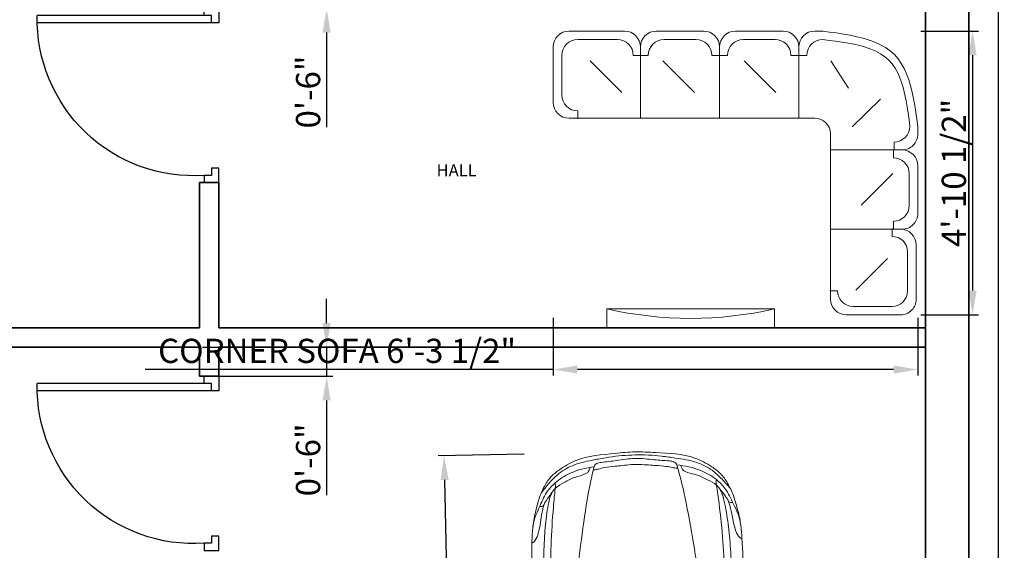
# Model space of a CAD drawing. Units: inches. Extents: x -24887 to 3061, y 1794 to 4919553.
# Tile 11 of 14: x 2858 to 3061, y 2080 to 2190. Entities that reach past the tile are written whole.
import ezdxf

# ---------------------------------------------------------------- set-up
doc = ezdxf.new("R2010")
doc.units = ezdxf.units.IN
for name, color, linetype, lineweight in [('A-ANNO-DIMS', 2, 'Continuous', 18), ('A-AREA-IDEN', 7, 'Continuous', 18), ('A-FLOR-PRKG', 8, 'Continuous', 13), ('A-FURN', 8, 'Continuous', 18), ('door', 4, 'Continuous', 25), ('TV', 210, 'Continuous', 18), ('wall', 7, 'Continuous', 35)]:
    doc.layers.add(name, color=color, linetype=linetype, lineweight=lineweight)
doc.styles.get("Standard").update_dxf_attribs({"font": 'arial.ttf'})
doc.dimstyles.new('ISO-25', dxfattribs={"dimtxt": 5, "dimasz": 5, "dimexe": 1.25, "dimexo": 0.625, "dimtad": 1, "dimdec": 1, "dimlunit": 3, "dimtxsty": 'Standard', "dimcen": 2.5, "dimadec": 0, "dimazin": 0, "dimtfac": 1, "dimtdec": 1, "dimtmove": 0, "dimatfit": 3, "dimfxl": 1, "dimarcsym": 0})

# ---------------------------------------------------------------- blocks, each defined once
blk = doc.blocks.new('A$C242571DA')
for points, knots in [([(0, 873.4), (0, 927.8), (15.6, 1088.6), (25.5, 1309.8), (120.7, 1476.4), (189.2, 1569), (273.5, 1623.1), (369.9, 1666.3), (483, 1694.7), (561.3, 1714.9), (604.6, 1715.7)], [0, 0, 0, 0, 0.16039, 0.479033, 0.632967, 0.722015, 0.817474, 0.927562, 1.03733, 1.167094, 1.167094, 1.167094, 1.167094]), ([(604.6, 1715.7), (545.5, 1714.5), (448.5, 1664.6), (320.8, 1610.6), (225.4, 1521.2), (147.3, 1390.5), (121.7, 1275.2), (113.6, 1208.7)], [0, 0, 0, 0, 0.1772572, 0.3124951, 0.4151678, 0.5597243, 0.7575412, 0.7575412, 0.7575412, 0.7575412]), ([(722.7, 1726.6), (720.8, 1714.9), (694.5, 1689.9), (643, 1671.8), (573.6, 1655.4), (508.5, 1647), (455.2, 1634.7), (428.7, 1627.3), (416.9, 1624.1)], [0, 0, 0, 0, 0.034703, 0.0959761, 0.1659336, 0.2471559, 0.2929944, 0.3295918, 0.3295918, 0.3295918, 0.3295918]), ([(604.6, 1715.7), (642.1, 1723.4), (788.5, 1729.2), (1039.3, 1732.2), (1344.5, 1729.9), (1542, 1733.1), (1633.8, 1733.7)], [0, 0, 0, 0, 0.114897, 0.437061, 0.754269, 1.029686, 1.029686, 1.029686, 1.029686]), ([(310.7, 1637.3), (282.5, 1613.7), (230.1, 1569.9), (148.7, 1486.2), (84.8, 1361.3), (60, 1219), (32.6, 1054.3), (25.1, 944.9), (25.1, 873.4)], [0, 0, 0, 0, 0.1095129, 0.2035347, 0.3452507, 0.5161382, 0.6275464, 0.8383798, 0.8383798, 0.8383798, 0.8383798]), ([(426.8, 1656.7), (428.5, 1646.6), (426.9, 1625), (399.8, 1616.6), (368.1, 1593.9), (328, 1564.6), (271.6, 1523.9), (237, 1451.9), (196.2, 1376.7), (183.8, 1314.9), (170, 1279.6), (157.2, 1254.2), (133.3, 1244.4), (118.6, 1242.9)], [0, 0, 0, 0, 0.0304541, 0.0502818, 0.0786089, 0.1479133, 0.1986294, 0.2831705, 0.3780326, 0.4523267, 0.4667809, 0.4902599, 0.5347198, 0.5347198, 0.5347198, 0.5347198]), ([(323.7, 1557.5), (344.8, 1571.9), (400.4, 1585.1), (516, 1606.8), (680.3, 1625.8), (885.4, 1635.7), (1116.8, 1642.2), (1346.1, 1644.2), (1504.7, 1644.7), (1574, 1645.7)], [0, 0, 0, 0, 0.076148, 0.165903, 0.355672, 0.569871, 0.782325, 1.050047, 1.257936, 1.257936, 1.257936, 1.257936]), ([(1317.4, 1579.7), (1227.8, 1586.1), (1036, 1584.8), (741.2, 1572.5), (486.1, 1553.3), (333.3, 1534.3), (283.3, 1528.5)], [0, 0, 0, 0, 0.269375, 0.574535, 0.885339, 1.036319, 1.036319, 1.036319, 1.036319]), ([(113.6, 1208.7), (215.2, 1238.6), (443.2, 1284.9), (788, 1338.7), (1029.5, 1370.7), (1146.4, 1378.6)], [0, 0, 0, 0, 0.317374, 0.69576, 1.04714, 1.04714, 1.04714, 1.04714]), ([(113.6, 1208.7), (103.3, 1207), (83.6, 1187.6), (76.5, 1122.2), (68.2, 1017.3), (53.4, 925), (53.4, 873.4)], [0, 0, 0, 0, 0.0314754, 0.0702057, 0.1915753, 0.3439346, 0.3439346, 0.3439346, 0.3439346]), ([(135.5, 1213.1), (139.1, 1211.8), (138.4, 1193.3), (132.6, 1168.3), (118.8, 1111.9), (115.6, 1058.9), (109, 974.6), (102.4, 920.1), (102.4, 873.4)], [0, 0, 0, 0, 0.0114788, 0.0403472, 0.0875838, 0.1755608, 0.1991501, 0.3369659, 0.3369659, 0.3369659, 0.3369659]), ([(0, 873.4), (0, 819), (15.6, 658.1), (25.5, 437), (120.7, 270.3), (189.2, 177.8), (273.5, 123.7), (369.9, 80.4), (483, 52), (561.3, 31.9), (604.6, 31)], [0, 0, 0, 0, 0.16039, 0.479033, 0.632967, 0.722015, 0.817474, 0.927562, 1.03733, 1.167094, 1.167094, 1.167094, 1.167094]), ([(310.7, 109.5), (282.5, 133.1), (230.1, 176.9), (148.7, 260.5), (84.8, 385.5), (60, 527.8), (32.6, 692.4), (25.1, 801.9), (25.1, 873.4)], [0, 0, 0, 0, 0.1095129, 0.2035347, 0.3452507, 0.5161382, 0.6275464, 0.8383798, 0.8383798, 0.8383798, 0.8383798]), ([(113.6, 538.1), (103.3, 539.8), (83.6, 559.2), (76.5, 624.5), (68.2, 729.4), (53.4, 821.7), (53.4, 873.4)], [0, 0, 0, 0, 0.0314754, 0.0702057, 0.1915753, 0.3439346, 0.3439346, 0.3439346, 0.3439346]), ([(135.5, 533.6), (139.1, 534.9), (138.4, 553.4), (132.6, 578.4), (118.8, 634.9), (115.6, 687.8), (109, 772.2), (102.4, 826.7), (102.4, 873.4)], [0, 0, 0, 0, 0.0114788, 0.0403472, 0.0875838, 0.1755608, 0.1991501, 0.3369659, 0.3369659, 0.3369659, 0.3369659]), ([(604.6, 31), (545.5, 32.3), (448.5, 82.2), (320.8, 136.1), (225.4, 225.5), (147.3, 356.2), (121.7, 471.5), (113.6, 538.1)], [0, 0, 0, 0, 0.1772572, 0.3124951, 0.4151678, 0.5597243, 0.7575412, 0.7575412, 0.7575412, 0.7575412]), ([(113.6, 538.1), (215.2, 508.2), (443.2, 461.9), (788, 408.1), (1029.5, 376), (1146.4, 368.2)], [0, 0, 0, 0, 0.317374, 0.69576, 1.04714, 1.04714, 1.04714, 1.04714]), ([(426.8, 90), (428.5, 100.2), (426.9, 121.8), (399.8, 130.1), (368.1, 152.8), (328, 182.2), (271.6, 222.8), (237, 294.9), (196.2, 370.1), (183.8, 431.9), (170, 467.2), (157.2, 492.6), (133.3, 502.4), (118.6, 503.9)], [0, 0, 0, 0, 0.0304541, 0.0502818, 0.0786089, 0.1479133, 0.1986294, 0.2831705, 0.3780326, 0.4523267, 0.4667809, 0.4902599, 0.5347198, 0.5347198, 0.5347198, 0.5347198]), ([(1317.4, 167), (1227.8, 160.7), (1036, 161.9), (741.2, 174.2), (486.1, 193.4), (333.3, 212.5), (283.3, 218.3)], [0, 0, 0, 0, 0.269375, 0.574535, 0.885339, 1.036319, 1.036319, 1.036319, 1.036319]), ([(323.7, 189.2), (344.8, 174.9), (400.4, 161.7), (516, 139.9), (680.3, 121), (885.4, 111), (1116.8, 104.5), (1346.1, 102.5), (1504.7, 102), (1574, 101.1)], [0, 0, 0, 0, 0.076148, 0.165903, 0.355672, 0.569871, 0.782325, 1.050047, 1.257936, 1.257936, 1.257936, 1.257936]), ([(722.7, 20.2), (720.8, 31.8), (694.5, 56.8), (643, 75), (573.6, 91.4), (508.5, 99.8), (455.2, 112.1), (428.7, 119.5), (416.9, 122.6)], [0, 0, 0, 0, 0.034703, 0.0959761, 0.1659336, 0.2471559, 0.2929944, 0.3295918, 0.3295918, 0.3295918, 0.3295918]), ([(604.6, 31), (642.1, 23.4), (788.5, 17.5), (1039.3, 14.6), (1344.5, 16.8), (1542, 13.6), (1633.8, 13.1)], [0, 0, 0, 0, 0.114897, 0.437061, 0.754269, 1.029686, 1.029686, 1.029686, 1.029686])]:
    blk.add_open_spline(points, degree=3, knots=knots)
for points in [[(283.3, 1528.5), (267.8, 1524.6), (251.4, 1527.5), (235.4, 1528.5)], [(283.3, 218.3), (267.8, 222.1), (251.4, 219.2), (235.4, 218.3)]]:
    blk.add_open_spline(points, degree=3)
blk = doc.blocks.new('A$C4B324E0D')
for points in [[(-0.4032, -0.0374), (-0.3959, 0.0153), (-0.3883, 0.0678), (-0.3801, 0.1195), (-0.3709, 0.1704), (-0.3605, 0.22), (-0.3485, 0.2679), (-0.3346, 0.314), (-0.3185, 0.3579), (-0.2998, 0.3993), (-0.2783, 0.4378), (-0.2537, 0.4731), (-0.2255, 0.5049), (-0.1936, 0.5331), (-0.1583, 0.5578), (-0.1198, 0.5793), (-0.0785, 0.5979), (-0.0346, 0.614), (0.0115, 0.628), (0.0595, 0.64), (0.1091, 0.6504), (0.1599, 0.6595), (0.2117, 0.6678), (0.2641, 0.6753), (0.3168, 0.6826)], [(0.3768, 0.6826), (0.3168, 0.6826)], [(0.9768, 0.6826), (0.6168, 0.6826)], [(1.5769, 0.6826), (1.2168, 0.6826)], [(1.8168, 0.6826), (2.2368, 0.6826)], [(-0.3432, -0.0374), (-0.3369, 0.0114), (-0.3303, 0.0599), (-0.3232, 0.1078), (-0.3151, 0.1548), (-0.3059, 0.2006), (-0.2951, 0.2449), (-0.2826, 0.2874), (-0.2681, 0.3278), (-0.2511, 0.3658), (-0.2315, 0.4011), (-0.2089, 0.4335), (-0.1831, 0.4625), (-0.1538, 0.488), (-0.1214, 0.5102), (-0.086, 0.5294), (-0.0479, 0.546), (-0.0075, 0.5602), (0.035, 0.5722), (0.0793, 0.5825), (0.125, 0.5914), (0.172, 0.599), (0.2198, 0.6057), (0.2682, 0.6119), (0.3168, 0.6177)], [(0.3168, 0.6177), (0.3168, 0.6177)], [(0.9168, 0.6177), (0.6768, 0.6177)], [(1.5168, 0.6177), (1.2768, 0.6177)], [(2.1704, 0.6177), (1.8704, 0.6177)], [(0.4968, 0.0226), (0.4968, 0.5626)], [(0.4968, 0.5626), (0.4968, 0.0226), (1.0968, 0.0226)], [(1.0968, 0.5626), (1.0968, 0.0226), (1.6968, 0.0226)], [(1.0968, 0.0226), (1.0968, 0.5626)], [(1.6968, 0.0226), (1.6968, 0.5626)], [(2.2368, 0.0226), (1.6968, 0.0226), (1.6968, 0.5626)], [(2.3569, 0.5626), (2.3569, 0.1426)], [(0.255, 0.4573), (0.1211, 0.2495)], [(0.4968, 0.4977), (0.4368, 0.4977), (0.4368, 0.4977)], [(0.5569, 0.4977), (0.5569, 0.4977), (0.4968, 0.4977)], [(0.9111, 0.4573), (0.6711, 0.2173)], [(1.0968, 0.4977), (1.0368, 0.4977), (1.0368, 0.4977)], [(1.1569, 0.4977), (1.1569, 0.4977), (1.0968, 0.4977)], [(1.527, 0.4573), (1.287, 0.2173)], [(1.6969, 0.4977), (1.6368, 0.4977), (1.6368, 0.4977)], [(1.7504, 0.4977), (1.7504, 0.4977), (1.6904, 0.4977)], [(2.0759, 0.4573), (1.8359, 0.2173)], [(2.2904, 0.1977), (2.2904, 0.4977)], [(-0.1199, 0.1664), (0.0943, -0.0414)], [(2.1704, 0.0177), (2.1704, 0.0777), (2.1704, 0.0777)], [(0.4968, 0.0226), (0.3768, 0.0226)], [(-0.4032, -0.0974), (-0.4032, -0.0374)], [(-0.3432, -0.0374), (-0.3432, -0.0374)], [(0.2568, -0.0974), (0.2568, -0.2174)], [(-0.2832, -0.8174), (0.2568, -0.8174), (0.2568, -0.2174)], [(0.2568, -0.2174), (-0.2832, -0.2174)], [(0.2568, -0.2174), (-0.2832, -0.2174)], [(-0.2232, -0.2174), (-0.2232, -0.1574), (-0.2232, -0.1574)], [(-0.2183, -0.2174), (-0.2183, -0.2774), (-0.2183, -0.2774)], [(-0.4032, -0.3374), (-0.4032, -0.6974)], [(-0.3383, -0.3974), (-0.3383, -0.6374)], [(-0.2136, -0.3946), (0.0264, -0.6346)], [(0.2568, -0.8174), (-0.2832, -0.8174)], [(-0.2732, -0.8174), (0.2568, -0.8174), (0.2568, -1.3475)], [(-0.2183, -0.7574), (-0.2183, -0.7574), (-0.2183, -0.8174)], [(-0.208, -0.8126), (-0.208, -0.8715), (-0.208, -0.8715)], [(0.2568, -0.8174), (0.2568, -1.3475)], [(-0.391, -1.3475), (-0.391, -0.9352)], [(-0.3258, -0.9893), (-0.3258, -1.2838)], [(-0.1734, -1.0387), (0.0666, -1.2787)], [(0.2043, -1.2838), (0.2043, -1.2838), (0.2632, -1.2838)], [(-0.208, -1.4016), (0.0865, -1.4016)], [(0.1391, -1.4653), (-0.2732, -1.4653)]]:
    blk.add_lwpolyline(points)
for centre, radius, start, end in [((0.3768, 0.5626), 0.12, 0, 90), ((0.6168, 0.5626), 0.12, 90, 180), ((0.9768, 0.5626), 0.12, 0, 90), ((1.2168, 0.5626), 0.12, 90, 180), ((1.5769, 0.5626), 0.12, 0, 90), ((1.8168, 0.5626), 0.12, 90, 180), ((2.2368, 0.5626), 0.12, 0, 90), ((0.3168, 0.4977), 0.12, 0, 90), ((0.6768, 0.4977), 0.12, 90, 180), ((0.9168, 0.4977), 0.12, 0, 90), ((1.2768, 0.4977), 0.12, 90, 180), ((1.5168, 0.4977), 0.12, 0, 90), ((1.8704, 0.4977), 0.12, 90, 180), ((2.1704, 0.4977), 0.12, 0, 90), ((2.1704, 0.1977), 0.12, 270, 0), ((2.2368, 0.1426), 0.12, 270, 0), ((0.3768, -0.0974), 0.12, 90, 180), ((-0.2232, -0.0374), 0.12, 180, 270), ((-0.2832, -0.0974), 0.12, 179.9997, 270), ((-0.2832, -0.3374), 0.12, 90, 180), ((-0.2183, -0.3974), 0.12, 90, 180), ((-0.2183, -0.6374), 0.12, 180, 270), ((-0.2832, -0.6974), 0.12, 179.9997, 270), ((-0.2732, -0.9352), 0.1178, 90, 180), ((-0.208, -0.9893), 0.1178, 90, 180), ((-0.208, -1.2838), 0.1178, 180, 270), ((0.0865, -1.2838), 0.1178, 270, 0), ((-0.2732, -1.3475), 0.1178, 179.9997, 270), ((0.1391, -1.3475), 0.1178, 270, 0)]:
    blk.add_arc(centre, radius, start, end)
blk = doc.blocks.new('A$C58C6152E')
at = {"xscale": 1.5, "yscale": 1.5, "zscale": 1.5, "rotation": 90}
blk.add_blockref('A$C4B324E0D', (1.024, 0.605), dxfattribs=at)
blk = doc.blocks.new('A$C15DC316E')
at = {"xscale": -1, "rotation": 270}
blk.add_blockref('A$C58C6152E', (0, 0), dxfattribs=at)
blk = doc.blocks.new('*D33')
at = {"layer": 'A-ANNO-DIMS', "color": 0, "lineweight": -2, "transparency": 16777216}
for p, q in [((3054.55, 2436.94), (3061.24, 2436.94)), ((3059.99, 2431.94), (3059.99, 1961.94)), ((3054.55, 1956.94), (3061.24, 1956.94))]:
    blk.add_line(p, q, dxfattribs=at)
at = {"layer": 'A-ANNO-DIMS', "color": 0, "transparency": 16777216}
for points in [[(3059.16, 2431.94), (3060.83, 2431.94), (3059.99, 2436.94)], [(3059.16, 1961.94), (3060.83, 1961.94), (3059.99, 1956.94)]]:
    blk.add_solid(points, dxfattribs=at)
at = {"layer": 'Defpoints', "color": 0, "transparency": 16777216}
for p in [(3053.93, 2436.94), (3053.93, 1956.94), (3059.99, 1956.94)]:
    blk.add_point(p, dxfattribs=at)
at = {"layer": 'A-ANNO-DIMS', "color": 0, "transparency": 16777216, "insert": (3056.82, 2196.94), "char_height": 5, "attachment_point": 5, "rotation": 90}
blk.add_mtext("40'", dxfattribs=at)
blk = doc.blocks.new('DOOR-SINGLE-36IN')
for p, q in [((34.5, 36), (37.5, 36)), ((34.5, 34.5), (34.5, 36)), ((37.5, 36), (37.5, 33)), ((36, 34.5), (34.5, 34.5)), ((36, 33), (36, 34.5)), ((37.5, 33), (36, 33)), ((36, 3), (0, 3)), ((37.5, 3), (36, 3)), ((36, 3), (36, 1.5)), ((37.5, 0), (37.5, 3)), ((36, 1.5), (0, 1.5)), ((36, 1.5), (34.5, 1.5)), ((34.5, 1.5), (34.5, 0)), ((34.5, 0), (37.5, 0))]:
    blk.add_line(p, q)
blk.add_arc((32.32, 2.25), 32.32, 86.1244, 181.3295)
blk = doc.blocks.new('*D62')
at = {"layer": 'A-ANNO-DIMS', "color": 0, "lineweight": -2, "transparency": 16777216}
for p, q in [((2962.02, 2099.85), (2944.25, 2099.49)), ((2945.61, 2094.52), (2947.76, 1990.25)), ((2964.37, 1985.59), (2946.61, 1985.22))]:
    blk.add_line(p, q, dxfattribs=at)
at = {"layer": 'A-ANNO-DIMS', "color": 0, "transparency": 16777216}
for points in [[(2946.44, 2094.53), (2944.77, 2094.5), (2945.5, 2099.51)], [(2948.59, 1990.27), (2946.92, 1990.23), (2947.86, 1985.25)]]:
    blk.add_solid(points, dxfattribs=at)
at = {"layer": 'Defpoints', "color": 0, "transparency": 16777216}
for p in [(2962.64, 2099.87), (2965, 1985.6), (2947.86, 1985.25)]:
    blk.add_point(p, dxfattribs=at)
at = {"layer": 'A-ANNO-DIMS', "color": 0, "transparency": 16777216, "insert": (2949.89, 2042.45), "char_height": 5, "attachment_point": 5, "rotation": 271.1816}
blk.add_mtext('CAR 9\'-6 1/2"', dxfattribs=at)
blk = doc.blocks.new('*D64')
at = {"layer": 'A-ANNO-DIMS', "color": 0, "lineweight": -2, "transparency": 16777216}
for p, q in [((2968.04, 2128.01), (2968.04, 2116.08)), ((3043.38, 2128.01), (3043.38, 2116.08)), ((2968.04, 2117.33), (2883.74, 2117.33)), ((3038.38, 2117.33), (2973.04, 2117.33))]:
    blk.add_line(p, q, dxfattribs=at)
at = {"layer": 'A-ANNO-DIMS', "color": 0, "transparency": 16777216}
for points in [[(2973.04, 2118.16), (2973.04, 2116.5), (2968.04, 2117.33)], [(3038.38, 2118.16), (3038.38, 2116.5), (3043.38, 2117.33)]]:
    blk.add_solid(points, dxfattribs=at)
at = {"layer": 'Defpoints', "color": 0, "transparency": 16777216}
for p in [(2968.04, 2128.63), (3043.38, 2128.63), (2968.04, 2117.33)]:
    blk.add_point(p, dxfattribs=at)
at = {"layer": 'A-ANNO-DIMS', "color": 0, "transparency": 16777216, "insert": (2923.39, 2120.54), "char_height": 5, "attachment_point": 5}
blk.add_mtext('CORNER SOFA 6\'-3 1/2"', dxfattribs=at)
blk = doc.blocks.new('*D65')
at = {"layer": 'A-ANNO-DIMS', "color": 0, "lineweight": -2, "transparency": 16777216}
for p, q in [((3044.01, 2187.26), (3055.93, 2187.26)), ((3054.68, 2182.26), (3054.68, 2133.63)), ((3044.01, 2128.63), (3055.93, 2128.63))]:
    blk.add_line(p, q, dxfattribs=at)
at = {"layer": 'A-ANNO-DIMS', "color": 0, "transparency": 16777216}
for points in [[(3053.85, 2182.26), (3055.52, 2182.26), (3054.68, 2187.26)], [(3053.85, 2133.63), (3055.52, 2133.63), (3054.68, 2128.63)]]:
    blk.add_solid(points, dxfattribs=at)
at = {"layer": 'Defpoints', "color": 0, "transparency": 16777216}
for p in [(3043.38, 2187.26), (3043.38, 2128.63), (3054.68, 2128.63)]:
    blk.add_point(p, dxfattribs=at)
at = {"layer": 'A-ANNO-DIMS', "color": 0, "transparency": 16777216, "insert": (3051.47, 2157.95), "char_height": 5, "attachment_point": 5, "rotation": 90}
blk.add_mtext('4\'-10 1/2"', dxfattribs=at)
blk = doc.blocks.new('*D114')
at = {"layer": 'A-ANNO-DIMS', "color": 0, "lineweight": -2, "transparency": 16777216}
for p, q in [((2921.23, 2202.94), (2921.23, 2207.94)), ((2895.55, 2197.94), (2922.48, 2197.94)), ((2921.23, 2197.94), (2921.23, 2191.94)), ((2895.55, 2191.94), (2922.48, 2191.94)), ((2921.23, 2186.94), (2921.23, 2167.4))]:
    blk.add_line(p, q, dxfattribs=at)
at = {"layer": 'A-ANNO-DIMS', "color": 0, "transparency": 16777216}
for points in [[(2920.39, 2202.94), (2922.06, 2202.94), (2921.23, 2197.94)], [(2920.39, 2186.94), (2922.06, 2186.94), (2921.23, 2191.94)]]:
    blk.add_solid(points, dxfattribs=at)
at = {"layer": 'Defpoints', "color": 0, "transparency": 16777216}
for p in [(2894.93, 2197.94), (2894.93, 2191.94), (2921.23, 2191.94)]:
    blk.add_point(p, dxfattribs=at)
at = {"layer": 'A-ANNO-DIMS', "color": 0, "transparency": 16777216, "insert": (2918.05, 2174.67), "char_height": 5, "attachment_point": 5, "rotation": 90}
blk.add_mtext('0\'-6"', dxfattribs=at)
blk = doc.blocks.new('*D115')
at = {"layer": 'A-ANNO-DIMS', "color": 0, "lineweight": -2, "transparency": 16777216}
for p, q in [((2921.23, 2126.94), (2921.23, 2131.94)), ((2895.55, 2121.94), (2922.48, 2121.94)), ((2921.23, 2121.94), (2921.23, 2115.94)), ((2895.55, 2115.94), (2922.48, 2115.94)), ((2921.23, 2110.94), (2921.23, 2091.4))]:
    blk.add_line(p, q, dxfattribs=at)
at = {"layer": 'A-ANNO-DIMS', "color": 0, "transparency": 16777216}
for points in [[(2920.39, 2126.94), (2922.06, 2126.94), (2921.23, 2121.94)], [(2920.39, 2110.94), (2922.06, 2110.94), (2921.23, 2115.94)]]:
    blk.add_solid(points, dxfattribs=at)
at = {"layer": 'Defpoints', "color": 0, "transparency": 16777216}
for p in [(2894.93, 2121.94), (2894.93, 2115.94), (2921.23, 2115.94)]:
    blk.add_point(p, dxfattribs=at)
at = {"layer": 'A-ANNO-DIMS', "color": 0, "transparency": 16777216, "insert": (2918.05, 2098.67), "char_height": 5, "attachment_point": 5, "rotation": 90}
blk.add_mtext('0\'-6"', dxfattribs=at)

msp = doc.modelspace()

# ---------------------------------------------------------------- linework, layer by layer
at = {"layer": 'TV'}
msp.add_lwpolyline([(2979.12, 2125.94), (3013.78, 2125.94), (3013.78, 2129.86), (2979.12, 2129.86)], close=True, dxfattribs=at)
msp.add_arc((2996.45, 2205.48), 77.58, 257.0921, 282.9079, dxfattribs=at)
at = {"layer": 'wall'}
for p, q in [((3053.93, 1956.94), (3053.93, 2436.94)), ((3044.93, 1965.94), (3044.93, 2427.94)), ((2894.93, 2155.94), (2898.93, 2155.94)), ((2894.93, 2155.94), (2894.93, 2125.94)), ((2898.93, 2155.94), (2898.93, 2125.94)), ((2894.93, 2125.94), (2762.93, 2125.94)), ((3044.93, 2125.94), (2898.93, 2125.94)), ((2894.93, 2121.94), (2762.93, 2121.94)), ((2894.93, 2121.94), (2894.93, 2115.94)), ((3044.93, 2121.94), (2898.93, 2121.94)), ((2898.93, 2121.94), (2898.93, 2115.94)), ((2894.93, 2115.94), (2898.93, 2115.94))]:
    msp.add_line(p, q, dxfattribs=at)

# ---------------------------------------------------------------- block references
at = {"layer": 'A-FLOR-PRKG', "xscale": 0.0254481748236463, "yscale": 0.0254481748236463, "zscale": 0.0254481748236463, "rotation": 271.1816230615127}
msp.add_blockref('A$C242571DA', (2962.75, 2099.87), dxfattribs=at)
at = {"layer": 'A-FURN', "xscale": 18.19849814291388, "yscale": 18.19849814291388, "zscale": 18.19849814291388, "rotation": 180}
msp.add_blockref('A$C15DC316E', (3043.38, 2187.26), dxfattribs=at)
at = {"layer": 'door', "extrusion": (0, 0, -1), "zscale": -1, "rotation": 180}
for p in [(-2861.43, 2191.94), (-2861.43, 2115.94)]:
    msp.add_blockref('DOOR-SINGLE-36IN', p, dxfattribs=at)

# ---------------------------------------------------------------- texts
at = {"layer": 'A-AREA-IDEN', "insert": (2943.96, 2159.73), "char_height": 2.5, "attachment_point": 1}
msp.add_mtext_dynamic_manual_height_columns('HALL', width=34.2323, gutter_width=12.5, heights=[0], dxfattribs=at)

# ---------------------------------------------------------------- dimensions: what is measured, and where the dimension line sits
at = {"layer": 'A-ANNO-DIMS'}
for base, p1, p2, angle, override, picture, middle in [((3059.99, 1956.94), (3053.93, 2436.94), (3053.93, 1956.94), 90, {"dimclrd": 0, "dimclre": 0, "dimclrt": 0}, '*D33', (3056.82, 2196.94)), ((2921.23, 2191.94), (2894.93, 2197.94), (2894.93, 2191.94), 270, {"dimdec": 1, "dimlfac": 1, "dimrnd": 0, "dimzin": 1, "dimdsep": 46, "dimlunit": 4, "dimfrac": 2}, '*D114', (2918.05, 2174.67)), ((3054.68, 2128.63), (3043.38, 2187.26), (3043.38, 2128.63), 270, {"dimdec": 1, "dimlfac": 1, "dimrnd": 0, "dimzin": 1, "dimdsep": 46, "dimlunit": 4, "dimfrac": 2}, '*D65', (3051.47, 2157.95)), ((2921.23, 2115.94), (2894.93, 2121.94), (2894.93, 2115.94), 270, {"dimdec": 1, "dimlfac": 1, "dimrnd": 0, "dimzin": 1, "dimdsep": 46, "dimlunit": 4, "dimfrac": 2}, '*D115', (2918.05, 2098.67))]:
    dim = msp.add_linear_dim(base=base, p1=p1, p2=p2, angle=angle, dimstyle='ISO-25', override=override, dxfattribs=at)
    dim.commit()
    dim.dimension.update_dxf_attribs({"geometry": picture, "text_midpoint": middle})
for base, p1, p2, angle, text, picture, middle in [((2968.04, 2117.33), (3043.38, 2128.63), (2968.04, 2128.63), 180, 'CORNER SOFA <>', '*D64', (2923.39, 2120.54)), ((2947.86, 1985.25), (2962.64, 2099.87), (2965, 1985.6), 271.1816, 'CAR <>', '*D62', (2949.89, 2042.45))]:
    dim = msp.add_linear_dim(base=base, p1=p1, p2=p2, angle=angle, text=text, dimstyle='ISO-25', override={"dimdec": 1, "dimlfac": 1, "dimrnd": 0, "dimzin": 1, "dimdsep": 46, "dimlunit": 4, "dimfrac": 2}, dxfattribs=at)
    dim.commit()
    dim.dimension.update_dxf_attribs({"geometry": picture, "text_midpoint": middle})

doc.saveas('drawing.dxf')
